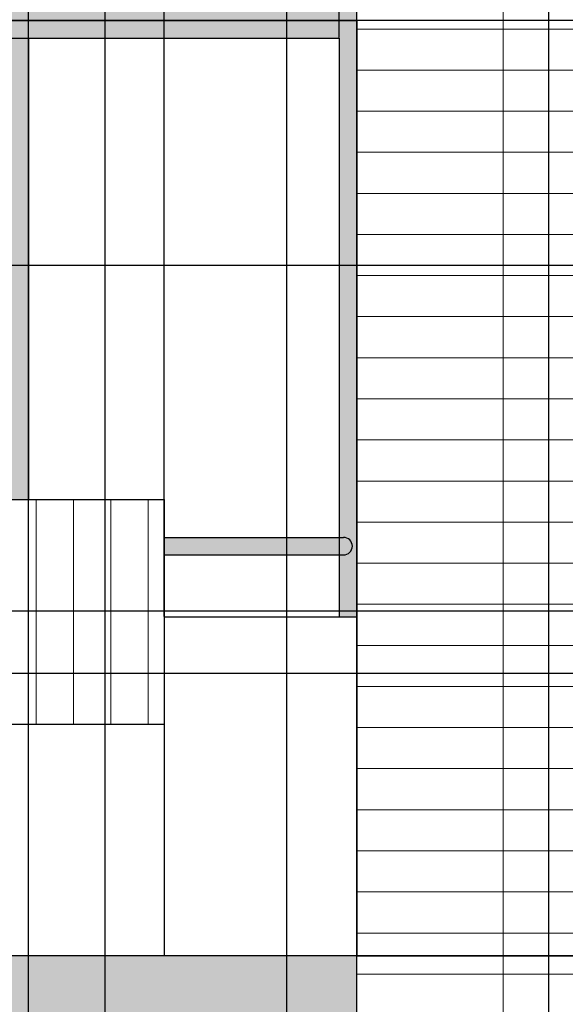
# Model space of a CAD drawing. Units: inches. Extents: x 241 to 943, y 109 to 1396.
# Tile 23 of 34: x 470 to 532, y 1065 to 1178. Entities that reach past the tile are written whole.
import ezdxf

# ---------------------------------------------------------------- set-up
doc = ezdxf.new("R2010")
doc.units = ezdxf.units.IN
doc.header["$MEASUREMENT"] = 0
for name, color, linetype, lineweight in [('A-ANNO-DIMS', 2, 'Continuous', 18), ('A-ELEV', 7, 'Continuous', 25), ('A-ELEV-SHAD', 9, 'Continuous', 13), ('A-GLAZ-PATT', 18, 'Continuous', 13), ('A-WALL-PATT', 8, 'Continuous', 13)]:
    doc.layers.add(name, color=color, linetype=linetype, lineweight=lineweight)
doc.styles.get("Standard").update_dxf_attribs({"font": 'arial.ttf'})
doc.dimstyles.get("Standard").update_dxf_attribs({"dimtxt": 1.4375, "dimasz": 0.18, "dimexe": 0.18, "dimexo": 0.0625, "dimgap": 0.09, "dimtad": 0, "dimtih": 1, "dimtoh": 1, "dimdec": 4, "dimzin": 0, "dimdsep": 46, "dimlunit": 4, "dimtxsty": 'Standard', "dimcen": 0.09, "dimadec": 0, "dimazin": 0, "dimtfac": 1, "dimtdec": 4, "dimtofl": 0, "dimtmove": 0, "dimatfit": 3, "dimfxl": 1, "dimtolj": 1, "dimtzin": 0, "dimarcsym": 0})

# ---------------------------------------------------------------- blocks, each defined once
blk = doc.blocks.new('BALCONY-RAIL')
for p, q in [((26.08, 26.37), (26.08, 52.06)), ((26.08, 52.06), (99.3, 52.06)), ((99.3, 52.06), (99.3, 26.37)), ((3.52, 47.73), (1, 47.73)), ((3.52, 47.73), (26.08, 47.73)), ((3.52, 45.73), (1, 45.73)), ((3.52, 45.73), (26.08, 45.73)), ((99.3, 26.37), (26.08, 26.37)), ((26.08, 26.37), (26.08, 0)), ((99.3, 26.37), (99.3, 0))]:
    blk.add_line(p, q)
blk.add_arc((1, 46.73), 1, 90, 270)
blk = doc.blocks.new('*D7')
at = {"layer": 'A-ANNO-DIMS', "color": 0, "lineweight": -2, "transparency": 16777216}
for p, q in [((508.24, 1336.12), (244.31, 1336.12)), ((244.49, 1335.94), (244.49, 753.25)), ((244.49, 168.92), (244.49, 751.6)), ((303.17, 168.74), (244.31, 168.74))]:
    blk.add_line(p, q, dxfattribs=at)
at = {"layer": 'A-ANNO-DIMS', "color": 0, "transparency": 16777216}
for points in [[(244.46, 1335.94), (244.52, 1335.94), (244.49, 1336.12)], [(244.46, 168.92), (244.52, 168.92), (244.49, 168.74)]]:
    blk.add_solid(points, dxfattribs=at)
at = {"layer": 'Defpoints', "color": 0, "transparency": 16777216}
for p in [(244.49, 1336.12), (508.31, 1336.12), (303.24, 168.74)]:
    blk.add_point(p, dxfattribs=at)
at = {"layer": 'A-ANNO-DIMS', "color": 0, "transparency": 16777216, "insert": (244.49, 752.43), "char_height": 1.438, "attachment_point": 5}
blk.add_mtext('\\A1;1167.4', dxfattribs=at)
blk = doc.blocks.new('*D10')
at = {"layer": 'A-ANNO-DIMS', "color": 0, "lineweight": -2, "transparency": 16777216}
for p, q in [((462.11, 384.24), (462.11, 1395.05)), ((462.29, 1394.87), (468.4, 1394.87)), ((479.42, 1394.87), (473.3, 1394.87)), ((479.6, 384.24), (479.6, 1395.05))]:
    blk.add_line(p, q, dxfattribs=at)
at = {"layer": 'A-ANNO-DIMS', "color": 0, "transparency": 16777216}
for points in [[(462.29, 1394.9), (462.29, 1394.84), (462.11, 1394.87)], [(479.42, 1394.9), (479.42, 1394.84), (479.6, 1394.87)]]:
    blk.add_solid(points, dxfattribs=at)
at = {"layer": 'Defpoints', "color": 0, "transparency": 16777216}
for p in [(479.6, 1394.87), (462.11, 384.18), (479.6, 384.18)]:
    blk.add_point(p, dxfattribs=at)
at = {"layer": 'A-ANNO-DIMS', "color": 0, "transparency": 16777216, "insert": (470.85, 1394.87), "char_height": 1.438, "attachment_point": 5}
blk.add_mtext('\\A1;17.49', dxfattribs=at)
blk = doc.blocks.new('*D11')
at = {"layer": 'A-ANNO-DIMS', "color": 0, "lineweight": -2, "transparency": 16777216}
for p, q in [((500.33, 384.24), (500.33, 1395.05)), ((500.51, 1394.87), (513.31, 1394.87)), ((530.05, 1394.87), (517.25, 1394.87)), ((530.23, 384.24), (530.23, 1395.05))]:
    blk.add_line(p, q, dxfattribs=at)
at = {"layer": 'A-ANNO-DIMS', "color": 0, "transparency": 16777216}
for points in [[(500.51, 1394.9), (500.51, 1394.84), (500.33, 1394.87)], [(530.05, 1394.9), (530.05, 1394.84), (530.23, 1394.87)]]:
    blk.add_solid(points, dxfattribs=at)
at = {"layer": 'Defpoints', "color": 0, "transparency": 16777216}
for p in [(530.23, 1394.87), (500.33, 384.18), (530.23, 384.18)]:
    blk.add_point(p, dxfattribs=at)
at = {"layer": 'A-ANNO-DIMS', "color": 0, "transparency": 16777216, "insert": (515.28, 1394.87), "char_height": 1.438, "attachment_point": 5}
blk.add_mtext('\\A1;29.9', dxfattribs=at)
blk = doc.blocks.new('*D12')
at = {"layer": 'A-ANNO-DIMS', "color": 0, "lineweight": -2, "transparency": 16777216}
for p, q in [((530.23, 384.24), (530.23, 1395.05)), ((530.41, 1394.87), (587.56, 1394.87)), ((650.73, 1394.87), (593.58, 1394.87)), ((650.91, 384.24), (650.91, 1395.05))]:
    blk.add_line(p, q, dxfattribs=at)
at = {"layer": 'A-ANNO-DIMS', "color": 0, "transparency": 16777216}
for points in [[(530.41, 1394.9), (530.41, 1394.84), (530.23, 1394.87)], [(650.73, 1394.9), (650.73, 1394.84), (650.91, 1394.87)]]:
    blk.add_solid(points, dxfattribs=at)
at = {"layer": 'Defpoints', "color": 0, "transparency": 16777216}
for p in [(650.91, 1394.87), (530.23, 384.18), (650.91, 384.18)]:
    blk.add_point(p, dxfattribs=at)
at = {"layer": 'A-ANNO-DIMS', "color": 0, "transparency": 16777216, "insert": (590.57, 1394.87), "char_height": 1.438, "attachment_point": 5}
blk.add_mtext('\\A1;120.68', dxfattribs=at)
blk = doc.blocks.new('*D49')
at = {"layer": 'A-ANNO-DIMS', "color": 0, "lineweight": -2, "transparency": 16777216}
for p, q in [((766.24, 1177.54), (244.31, 1177.54)), ((244.49, 1177.36), (244.49, 1141.12)), ((244.49, 1103.23), (244.49, 1139.47)), ((766.24, 1103.05), (244.31, 1103.05))]:
    blk.add_line(p, q, dxfattribs=at)
at = {"layer": 'A-ANNO-DIMS', "color": 0, "transparency": 16777216}
for points in [[(244.46, 1177.36), (244.52, 1177.36), (244.49, 1177.54)], [(244.46, 1103.23), (244.52, 1103.23), (244.49, 1103.05)]]:
    blk.add_solid(points, dxfattribs=at)
at = {"layer": 'Defpoints', "color": 0, "transparency": 16777216}
for p in [(244.49, 1177.54), (766.3, 1177.54), (766.3, 1103.05)]:
    blk.add_point(p, dxfattribs=at)
at = {"layer": 'A-ANNO-DIMS', "color": 0, "transparency": 16777216, "insert": (244.49, 1140.29), "char_height": 1.438, "attachment_point": 5}
blk.add_mtext('\\A1;74.49', dxfattribs=at)
blk = doc.blocks.new('*D57')
at = {"layer": 'A-ANNO-DIMS', "color": 0, "lineweight": -2, "transparency": 16777216}
for p, q in [((508.31, 1070.92), (508.31, 1395.05)), ((508.49, 1394.87), (518.04, 1394.87)), ((533.77, 1394.87), (524.21, 1394.87)), ((533.95, 1108.23), (533.95, 1395.05))]:
    blk.add_line(p, q, dxfattribs=at)
at = {"layer": 'A-ANNO-DIMS', "color": 0, "transparency": 16777216}
for points in [[(508.49, 1394.9), (508.49, 1394.84), (508.31, 1394.87)], [(533.77, 1394.9), (533.77, 1394.84), (533.95, 1394.87)]]:
    blk.add_solid(points, dxfattribs=at)
at = {"layer": 'Defpoints', "color": 0, "transparency": 16777216}
for p in [(533.95, 1394.87), (533.95, 1108.17), (508.31, 1070.85)]:
    blk.add_point(p, dxfattribs=at)
at = {"layer": 'A-ANNO-DIMS', "color": 0, "transparency": 16777216, "insert": (521.13, 1394.87), "char_height": 1.438, "attachment_point": 5}
blk.add_mtext('\\A1;25.646', dxfattribs=at)
blk = doc.blocks.new('*D59')
at = {"layer": 'A-ANNO-DIMS', "color": 0, "lineweight": -2, "transparency": 16777216}
for p, q in [((398.31, 1175.6), (398.31, 1395.05)), ((398.49, 1394.87), (450.7, 1394.87)), ((506.13, 1394.87), (453.92, 1394.87)), ((506.31, 1175.6), (506.31, 1395.05))]:
    blk.add_line(p, q, dxfattribs=at)
at = {"layer": 'A-ANNO-DIMS', "color": 0, "transparency": 16777216}
for points in [[(398.49, 1394.9), (398.49, 1394.84), (398.31, 1394.87)], [(506.13, 1394.9), (506.13, 1394.84), (506.31, 1394.87)]]:
    blk.add_solid(points, dxfattribs=at)
at = {"layer": 'Defpoints', "color": 0, "transparency": 16777216}
for p in [(506.31, 1394.87), (398.31, 1175.54), (506.31, 1175.54)]:
    blk.add_point(p, dxfattribs=at)
at = {"layer": 'A-ANNO-DIMS', "color": 0, "transparency": 16777216, "insert": (452.31, 1394.87), "char_height": 1.438, "attachment_point": 5}
blk.add_mtext('\\A1;108', dxfattribs=at)
blk = doc.blocks.new('*D62')
at = {"layer": 'A-ANNO-DIMS', "color": 0, "lineweight": -2, "transparency": 16777216}
for p, q in [((424.11, 568.89), (424.11, 1395.05)), ((424.29, 1394.87), (492.35, 1394.87)), ((565.02, 1394.87), (496.96, 1394.87)), ((565.2, 568.89), (565.2, 1395.05))]:
    blk.add_line(p, q, dxfattribs=at)
at = {"layer": 'A-ANNO-DIMS', "color": 0, "transparency": 16777216}
for points in [[(424.29, 1394.9), (424.29, 1394.84), (424.11, 1394.87)], [(565.02, 1394.9), (565.02, 1394.84), (565.2, 1394.87)]]:
    blk.add_solid(points, dxfattribs=at)
at = {"layer": 'Defpoints', "color": 0, "transparency": 16777216}
for p in [(565.2, 1394.87), (424.11, 568.83), (565.2, 568.83)]:
    blk.add_point(p, dxfattribs=at)
at = {"layer": 'A-ANNO-DIMS', "color": 0, "transparency": 16777216, "insert": (494.66, 1394.87), "char_height": 1.438, "attachment_point": 5}
blk.add_mtext('\\A1;141.1', dxfattribs=at)
blk = doc.blocks.new('*D65')
at = {"layer": 'A-ANNO-DIMS', "color": 0, "lineweight": -2, "transparency": 16777216}
for p, q in [((424.11, 700.85), (424.11, 1395.05)), ((424.29, 1394.87), (505.52, 1394.87)), ((592.77, 1394.87), (511.54, 1394.87)), ((592.95, 700.85), (592.95, 1395.05))]:
    blk.add_line(p, q, dxfattribs=at)
at = {"layer": 'A-ANNO-DIMS', "color": 0, "transparency": 16777216}
for points in [[(424.29, 1394.9), (424.29, 1394.84), (424.11, 1394.87)], [(592.77, 1394.9), (592.77, 1394.84), (592.95, 1394.87)]]:
    blk.add_solid(points, dxfattribs=at)
at = {"layer": 'Defpoints', "color": 0, "transparency": 16777216}
for p in [(592.95, 1394.87), (424.11, 700.79), (592.95, 700.79)]:
    blk.add_point(p, dxfattribs=at)
at = {"layer": 'A-ANNO-DIMS', "color": 0, "transparency": 16777216, "insert": (508.53, 1394.87), "char_height": 1.438, "attachment_point": 5}
blk.add_mtext('\\A1;168.85', dxfattribs=at)
blk = doc.blocks.new('*D67')
at = {"layer": 'A-ANNO-DIMS', "color": 0, "lineweight": -2, "transparency": 16777216}
for p, q in [((389.04, 773.55), (389.04, 1395.05)), ((389.22, 1394.87), (495.34, 1394.87)), ((607.64, 1394.87), (501.52, 1394.87)), ((607.82, 773.55), (607.82, 1395.05))]:
    blk.add_line(p, q, dxfattribs=at)
at = {"layer": 'A-ANNO-DIMS', "color": 0, "transparency": 16777216}
for points in [[(389.22, 1394.9), (389.22, 1394.84), (389.04, 1394.87)], [(607.64, 1394.9), (607.64, 1394.84), (607.82, 1394.87)]]:
    blk.add_solid(points, dxfattribs=at)
at = {"layer": 'Defpoints', "color": 0, "transparency": 16777216}
for p in [(607.82, 1394.87), (389.04, 773.49), (607.82, 773.49)]:
    blk.add_point(p, dxfattribs=at)
at = {"layer": 'A-ANNO-DIMS', "color": 0, "transparency": 16777216, "insert": (498.43, 1394.87), "char_height": 1.438, "attachment_point": 5}
blk.add_mtext('\\A1;218.77', dxfattribs=at)
blk = doc.blocks.new('*D69')
at = {"layer": 'A-ANNO-DIMS', "color": 0, "lineweight": -2, "transparency": 16777216}
for p, q in [((389.04, 941.55), (389.04, 1395.05)), ((389.22, 1394.87), (476.28, 1394.87)), ((567.95, 1394.87), (480.9, 1394.87)), ((568.13, 941.55), (568.13, 1395.05))]:
    blk.add_line(p, q, dxfattribs=at)
at = {"layer": 'A-ANNO-DIMS', "color": 0, "transparency": 16777216}
for points in [[(389.22, 1394.9), (389.22, 1394.84), (389.04, 1394.87)], [(567.95, 1394.9), (567.95, 1394.84), (568.13, 1394.87)]]:
    blk.add_solid(points, dxfattribs=at)
at = {"layer": 'Defpoints', "color": 0, "transparency": 16777216}
for p in [(568.13, 1394.87), (389.04, 941.49), (568.13, 941.49)]:
    blk.add_point(p, dxfattribs=at)
at = {"layer": 'A-ANNO-DIMS', "color": 0, "transparency": 16777216, "insert": (478.59, 1394.87), "char_height": 1.438, "attachment_point": 5}
blk.add_mtext('\\A1;179.1', dxfattribs=at)
blk = doc.blocks.new('*D72')
at = {"layer": 'A-ANNO-DIMS', "color": 0, "lineweight": -2, "transparency": 16777216}
for p, q in [((389.04, 1109.55), (389.04, 1395.05)), ((389.22, 1394.87), (435.74, 1394.87)), ((486.16, 1394.87), (439.65, 1394.87)), ((486.34, 1109.55), (486.34, 1395.05))]:
    blk.add_line(p, q, dxfattribs=at)
at = {"layer": 'A-ANNO-DIMS', "color": 0, "transparency": 16777216}
for points in [[(389.22, 1394.9), (389.22, 1394.84), (389.04, 1394.87)], [(486.16, 1394.9), (486.16, 1394.84), (486.34, 1394.87)]]:
    blk.add_solid(points, dxfattribs=at)
at = {"layer": 'Defpoints', "color": 0, "transparency": 16777216}
for p in [(486.34, 1394.87), (389.04, 1109.49), (486.34, 1109.49)]:
    blk.add_point(p, dxfattribs=at)
at = {"layer": 'A-ANNO-DIMS', "color": 0, "transparency": 16777216, "insert": (437.69, 1394.87), "char_height": 1.438, "attachment_point": 5}
blk.add_mtext('\\A1;97.3', dxfattribs=at)
blk = doc.blocks.new('*D79')
at = {"layer": 'A-ANNO-DIMS', "color": 0, "lineweight": -2, "transparency": 16777216}
for p, q in [((479.6, 384.24), (479.6, 1395.05)), ((479.78, 1394.87), (486.88, 1394.87)), ((500.15, 1394.87), (493.05, 1394.87)), ((500.33, 384.24), (500.33, 1395.05))]:
    blk.add_line(p, q, dxfattribs=at)
at = {"layer": 'A-ANNO-DIMS', "color": 0, "transparency": 16777216}
for points in [[(479.78, 1394.9), (479.78, 1394.84), (479.6, 1394.87)], [(500.15, 1394.9), (500.15, 1394.84), (500.33, 1394.87)]]:
    blk.add_solid(points, dxfattribs=at)
at = {"layer": 'Defpoints', "color": 0, "transparency": 16777216}
for p in [(500.33, 1394.87), (479.6, 384.18), (500.33, 384.18)]:
    blk.add_point(p, dxfattribs=at)
at = {"layer": 'A-ANNO-DIMS', "color": 0, "transparency": 16777216, "insert": (489.96, 1394.87), "char_height": 1.438, "attachment_point": 5}
blk.add_mtext('\\A1;20.736', dxfattribs=at)
blk = doc.blocks.new('*D89')
at = {"layer": 'A-ANNO-DIMS', "color": 0, "lineweight": -2, "transparency": 16777216}
for p, q in [((377.04, 841.6), (377.04, 1395.05)), ((377.22, 1394.87), (494.32, 1394.87)), ((617.58, 1394.87), (500.48, 1394.87)), ((617.76, 841.6), (617.76, 1395.05))]:
    blk.add_line(p, q, dxfattribs=at)
at = {"layer": 'A-ANNO-DIMS', "color": 0, "transparency": 16777216}
for points in [[(377.22, 1394.9), (377.22, 1394.84), (377.04, 1394.87)], [(617.58, 1394.9), (617.58, 1394.84), (617.76, 1394.87)]]:
    blk.add_solid(points, dxfattribs=at)
at = {"layer": 'Defpoints', "color": 0, "transparency": 16777216}
for p in [(617.76, 1394.87), (377.04, 841.54), (617.76, 841.54)]:
    blk.add_point(p, dxfattribs=at)
at = {"layer": 'A-ANNO-DIMS', "color": 0, "transparency": 16777216, "insert": (497.4, 1394.87), "char_height": 1.438, "attachment_point": 5}
blk.add_mtext('\\A1;240.72', dxfattribs=at)
blk = doc.blocks.new('*D92')
at = {"layer": 'A-ANNO-DIMS', "color": 0, "lineweight": -2, "transparency": 16777216}
for p, q in [((508.24, 1336.12), (244.31, 1336.12)), ((244.49, 1335.94), (244.49, 1204.31)), ((244.49, 1071.03), (244.49, 1202.66)), ((508.24, 1070.85), (244.31, 1070.85))]:
    blk.add_line(p, q, dxfattribs=at)
at = {"layer": 'A-ANNO-DIMS', "color": 0, "transparency": 16777216}
for points in [[(244.46, 1335.94), (244.52, 1335.94), (244.49, 1336.12)], [(244.46, 1071.03), (244.52, 1071.03), (244.49, 1070.85)]]:
    blk.add_solid(points, dxfattribs=at)
at = {"layer": 'Defpoints', "color": 0, "transparency": 16777216}
for p in [(244.49, 1336.12), (508.31, 1336.12), (508.31, 1070.85)]:
    blk.add_point(p, dxfattribs=at)
at = {"layer": 'A-ANNO-DIMS', "color": 0, "transparency": 16777216, "insert": (244.49, 1203.48), "char_height": 1.438, "attachment_point": 5}
blk.add_mtext('\\A1;265.26', dxfattribs=at)
blk = doc.blocks.new('*D95')
at = {"layer": 'A-ANNO-DIMS', "color": 0, "lineweight": -2, "transparency": 16777216}
for p, q in [((724.88, 1108.17), (940.6, 1108.17)), ((940.42, 1107.99), (940.42, 1090.34)), ((940.42, 1071.03), (940.42, 1088.69)), ((508.37, 1070.85), (940.6, 1070.85))]:
    blk.add_line(p, q, dxfattribs=at)
at = {"layer": 'A-ANNO-DIMS', "color": 0, "transparency": 16777216}
for points in [[(940.39, 1107.99), (940.45, 1107.99), (940.42, 1108.17)], [(940.39, 1071.03), (940.45, 1071.03), (940.42, 1070.85)]]:
    blk.add_solid(points, dxfattribs=at)
at = {"layer": 'Defpoints', "color": 0, "transparency": 16777216}
for p in [(724.82, 1108.17), (940.42, 1108.17), (508.31, 1070.85)]:
    blk.add_point(p, dxfattribs=at)
at = {"layer": 'A-ANNO-DIMS', "color": 0, "transparency": 16777216, "insert": (940.42, 1089.51), "char_height": 1.438, "attachment_point": 5}
blk.add_mtext('\\A1;37.315', dxfattribs=at)
blk = doc.blocks.new('*D99')
at = {"layer": 'A-ANNO-DIMS', "color": 0, "lineweight": -2, "transparency": 16777216}
for p, q in [((417.09, 181.71), (417.09, 1395.05)), ((417.27, 1394.87), (539.16, 1394.87)), ((667.21, 1394.87), (545.33, 1394.87)), ((667.39, 214.58), (667.39, 1395.05))]:
    blk.add_line(p, q, dxfattribs=at)
at = {"layer": 'A-ANNO-DIMS', "color": 0, "transparency": 16777216}
for points in [[(417.27, 1394.9), (417.27, 1394.84), (417.09, 1394.87)], [(667.21, 1394.9), (667.21, 1394.84), (667.39, 1394.87)]]:
    blk.add_solid(points, dxfattribs=at)
at = {"layer": 'Defpoints', "color": 0, "transparency": 16777216}
for p in [(667.39, 1394.87), (667.39, 214.52), (417.09, 181.65)]:
    blk.add_point(p, dxfattribs=at)
at = {"layer": 'A-ANNO-DIMS', "color": 0, "transparency": 16777216, "insert": (542.24, 1394.87), "char_height": 1.438, "attachment_point": 5}
blk.add_mtext('\\A1;250.30', dxfattribs=at)
blk = doc.blocks.new('*D103')
at = {"layer": 'A-ANNO-DIMS', "color": 0, "lineweight": -2, "transparency": 16777216}
for p, q in [((470.87, 1007.6), (470.87, 1395.05)), ((471.05, 1394.87), (487.08, 1394.87)), ((508.13, 1394.87), (492.1, 1394.87)), ((508.31, 1009.6), (508.31, 1395.05))]:
    blk.add_line(p, q, dxfattribs=at)
at = {"layer": 'A-ANNO-DIMS', "color": 0, "transparency": 16777216}
for points in [[(471.05, 1394.9), (471.05, 1394.84), (470.87, 1394.87)], [(508.13, 1394.9), (508.13, 1394.84), (508.31, 1394.87)]]:
    blk.add_solid(points, dxfattribs=at)
at = {"layer": 'Defpoints', "color": 0, "transparency": 16777216}
for p in [(508.31, 1394.87), (508.31, 1009.54), (470.87, 1007.54)]:
    blk.add_point(p, dxfattribs=at)
at = {"layer": 'A-ANNO-DIMS', "color": 0, "transparency": 16777216, "insert": (489.59, 1394.87), "char_height": 1.438, "attachment_point": 5}
blk.add_mtext('\\A1;37.44', dxfattribs=at)
blk = doc.blocks.new('*D110')
at = {"layer": 'A-ANNO-DIMS', "color": 0, "lineweight": -2, "transparency": 16777216}
for p, q in [((535.89, 1149.58), (244.31, 1149.58)), ((244.49, 1149.4), (244.49, 1130.7)), ((244.49, 1110.35), (244.49, 1129.05)), ((535.89, 1110.17), (244.31, 1110.17))]:
    blk.add_line(p, q, dxfattribs=at)
at = {"layer": 'A-ANNO-DIMS', "color": 0, "transparency": 16777216}
for points in [[(244.46, 1149.4), (244.52, 1149.4), (244.49, 1149.58)], [(244.46, 1110.35), (244.52, 1110.35), (244.49, 1110.17)]]:
    blk.add_solid(points, dxfattribs=at)
at = {"layer": 'Defpoints', "color": 0, "transparency": 16777216}
for p in [(244.49, 1149.58), (535.95, 1149.58), (535.95, 1110.17)]:
    blk.add_point(p, dxfattribs=at)
at = {"layer": 'A-ANNO-DIMS', "color": 0, "transparency": 16777216, "insert": (244.49, 1129.87), "char_height": 1.438, "attachment_point": 5}
blk.add_mtext('\\A1;39.41', dxfattribs=at)

msp = doc.modelspace()

# ---------------------------------------------------------------- hatches: boundary and pattern name
at = {"layer": 'A-ELEV-SHAD'}
h = msp.add_hatch(color=256, dxfattribs=at)
h.dxf.hatch_style = 1
h.paths.add_polyline_path([(508.3064, 1070.8538), (377.0391, 1070.8538), (377.0391, 1009.5382), (508.3064, 1009.5382)])
h.paths.add_polyline_path([(508.3064, 1238.8538), (377.0391, 1238.8538), (377.0391, 1177.5382), (508.3064, 1177.5382)])
h.paths.add_polyline_path([(581.3632, 902.8538), (568.1348, 902.8538), (553.5166, 902.8538), (377.0391, 902.8538), (377.0391, 841.5382), (553.5166, 841.5382), (564.8076, 841.5382), (581.3632, 841.5382)])
h.paths.add_polyline_path([(820.8374, 1275.9142), (747.7579, 1275.9142), (747.7579, 1238.8538), (820.8374, 1238.8538)])
h.paths.add_polyline_path([(820.8374, 1238.8538), (747.7579, 1238.8538), (747.9341, 1223.0633), (820.8374, 1223.0633)])
h.paths.add_polyline_path([(396.3125, 841.5382), (377.0391, 841.5382), (377.0391, 734.8538), (389.0429, 734.8538), (389.0429, 735.188), (389.0429, 773.4916), (396.3125, 773.4916), (396.3125, 780.5808), (390.5597, 780.5808), (388.0428, 780.5808, -1), (388.0428, 782.5808), (390.5597, 782.5808), (396.3125, 782.5808)])
h = msp.add_hatch(color=256, dxfattribs=at)
h.dxf.hatch_style = 1
h.paths.add_polyline_path([(537.4269, 698.7912), (534.1778, 698.7912), (534.1778, 659.3434), (537.4269, 659.3434)])
h.paths.add_polyline_path([(508.0803, 698.7912), (450.9259, 698.7912), (450.9259, 659.3434), (452.9259, 659.3434), (452.9259, 696.7912), (506.0803, 696.7912), (506.0803, 659.3434), (508.0803, 659.3434)])
h.paths.add_polyline_path([(481.5031, 696.7912), (479.5031, 696.7912), (479.5031, 659.3434), (481.5031, 659.3434)], flags=17)
h.paths.add_polyline_path([(481.5031, 657.3434), (479.5031, 657.3434), (479.5031, 653.3371), (481.5031, 653.3371)], flags=17)
h.paths.add_polyline_path([(508.0803, 657.3434), (506.0803, 657.3434), (506.0803, 653.3371), (452.9259, 653.3371), (452.9259, 657.3434), (450.9259, 657.3434), (450.9259, 651.3371), (508.0803, 651.3371)])
h.paths.add_polyline_path([(428.1173, 839.5382), (426.1173, 839.5382), (426.1173, 786.9154), (428.1173, 786.9154)], flags=17)
h.paths.add_polyline_path([(470.8692, 839.5382), (468.8692, 839.5382), (468.8692, 786.9154), (470.8692, 786.9154)], flags=17)
h.paths.add_polyline_path([(508.3064, 841.5382), (396.3125, 841.5382), (396.3125, 782.5808), (398.3125, 782.5808), (398.3125, 839.5382), (506.3064, 839.5382), (506.3064, 782.5808), (508.3064, 782.5808)])
h.paths.add_polyline_path([(398.3125, 780.5808), (396.3125, 780.5808), (396.3125, 773.4916), (398.3125, 773.4916)])
h.paths.add_polyline_path([(508.3064, 780.5808), (506.3064, 780.5808), (506.3064, 773.4916), (508.3064, 773.4916)])
h.paths.add_polyline_path([(715.6236, 841.5382), (678.2674, 841.5382), (678.2674, 734.8538), (715.6236, 734.8538)])
h.paths.add_polyline_path([(680.2674, 839.5382), (682.4526, 839.5382), (713.6236, 839.5382), (713.6236, 736.9235), (690.2047, 736.9235), (680.2674, 736.9235)], flags=16)
h.paths.add_polyline_path([(792.691, 841.5382), (747.7579, 841.5382), (747.7579, 734.8538), (754.5373, 734.8538), (754.5373, 736.9235), (754.5373, 839.5382), (756.7224, 839.5382), (787.8934, 839.5382), (787.8934, 765.9585), (792.691, 765.9585)])
h.paths.add_polyline_path([(659.2925, 1009.5382), (657.2925, 1009.5382), (657.2925, 902.8538), (659.2925, 902.8538)])
h.paths.add_polyline_path([(751.5078, 976.6275), (712.5839, 976.6275), (712.5839, 974.6275), (751.5078, 974.6275)])
h.paths.add_polyline_path([(470.8692, 1007.5382), (468.8692, 1007.5382), (468.8692, 954.9154), (470.8692, 954.9154)], flags=17)
h.paths.add_polyline_path([(508.3064, 1009.5382), (396.3125, 1009.5382), (396.3125, 950.5808), (398.3125, 950.5808), (398.3125, 1007.5382), (506.3064, 1007.5382), (506.3064, 950.5808), (508.3064, 950.5808)])
h.paths.add_polyline_path([(428.1173, 1007.5382), (426.1173, 1007.5382), (426.1173, 954.9154), (428.1173, 954.9154)], flags=17)
h.paths.add_polyline_path([(398.3125, 948.5808), (396.3125, 948.5808), (396.3125, 941.4916), (398.3125, 941.4916)])
h.paths.add_polyline_path([(508.3064, 948.5808), (506.3064, 948.5808), (506.3064, 941.4916), (508.3064, 941.4916)])
h.paths.add_polyline_path([(428.1173, 1175.5382), (426.1173, 1175.5382), (426.1173, 1122.9154), (428.1173, 1122.9154)], flags=17)
h.paths.add_polyline_path([(508.3064, 1177.5382), (396.3125, 1177.5382), (396.3125, 1118.5808), (398.3125, 1118.5808), (398.3125, 1175.5382), (506.3064, 1175.5382), (506.3064, 1118.5808), (506.8039, 1118.5808, -1), (506.8039, 1116.5808), (506.3064, 1116.5808), (506.3064, 1109.4916), (508.3064, 1109.4916)])
h.paths.add_polyline_path([(470.8692, 1175.5382), (468.8692, 1175.5382), (468.8692, 1122.9154), (470.8692, 1122.9154)], flags=17)
h.paths.add_polyline_path([(398.3125, 1116.5808), (396.3125, 1116.5808), (396.3125, 1109.4916), (398.3125, 1109.4916)], flags=17)
h.paths.add_polyline_path([(724.819, 1177.7336), (533.952, 1177.7336), (533.952, 1108.1686), (724.819, 1108.1686)])
h.paths.add_polyline_path([(535.952, 1175.7336), (722.819, 1175.7336), (722.819, 1110.1686), (535.952, 1110.1686)], flags=0)
h.paths.add_polyline_path([(622.521, 1136.0739), (643.4534, 1136.0739), (643.4534, 1134.0739), (622.521, 1134.0739)], flags=0)
h.paths.add_polyline_path([(722.819, 1175.7336), (535.952, 1175.7336), (535.952, 1110.1686), (722.819, 1110.1686)], flags=16)
h.paths.add_polyline_path([(565.947, 1151.5772), (535.952, 1151.5772), (535.952, 1149.5772), (565.947, 1149.5772)], flags=0)
at = {"layer": 'A-GLAZ-PATT'}
h = msp.add_hatch(dxfattribs=at)
h.set_pattern_fill('ANSI31', color=256, scale=34, angle=45)
h.paths.add_polyline_path([(486.3418, 786.9154), (413.1187, 786.9154), (413.1187, 761.2284), (486.3418, 761.2284)])
h.paths.add_polyline_path([(486.3418, 954.9154), (413.1187, 954.9154), (413.1187, 929.2284), (486.3418, 929.2284)])
h.paths.add_polyline_path([(462.1074, 289.6933), (390.895, 289.6933), (390.895, 277.4626), (390.895, 274.3507), (462.1074, 274.3507), (462.1074, 277.4626)])
h.paths.add_polyline_path([(500.3323, 289.6933), (479.596, 289.6933), (479.596, 274.3507), (500.3323, 274.3507)])
h.paths.add_polyline_path([(450.9259, 566.8295), (426.1086, 566.8295), (426.1086, 498.4395), (446.4348, 498.4395), (446.4348, 519.3754), (450.9259, 519.3754), (450.9259, 525.3816), (445.5808, 525.3816, -1), (445.5808, 527.3816), (450.9259, 527.3816)])
h.paths.add_polyline_path([(563.2023, 508.9074), (534.1778, 508.9074), (508.1906, 508.9074), (508.1906, 498.4395), (563.2023, 498.4395)])
h.paths.add_polyline_path([(747.6328, 700.7912), (712.0171, 700.7912), (712.0171, 628.4013), (747.6328, 628.4013)])
h.paths.add_polyline_path([(446.4348, 643.7483), (426.1086, 643.7483), (426.1086, 630.4013), (446.4348, 630.4013)])
h.paths.add_polyline_path([(564.8076, 841.5382), (553.5166, 841.5382), (508.3064, 841.5382), (508.3064, 782.5808), (564.8076, 782.5808)])
h.paths.add_polyline_path([(564.8076, 780.5808), (508.3064, 780.5808), (508.3064, 773.4916), (564.8076, 773.4916)])
h.paths.add_polyline_path([(792.691, 762.5799), (759.6248, 762.5799), (759.6248, 736.9235), (759.6248, 734.8538), (792.691, 734.8538)])
h.paths.add_polyline_path([(564.8076, 1009.5382), (553.5166, 1009.5382), (508.3064, 1009.5382), (508.3064, 950.5808), (562.3033, 950.5808, -1), (562.3033, 948.5808), (508.3064, 948.5808), (508.3064, 941.4916), (564.8076, 941.4916)])
h.paths.add_polyline_path([(486.3418, 1122.9154), (413.1187, 1122.9154), (413.1187, 1097.2284), (486.3418, 1097.2284)])
h = msp.add_hatch(color=256, dxfattribs=at)
h.dxf.hatch_style = 1
h.paths.add_polyline_path([(396.3125, 1118.5808), (390.5597, 1118.5808), (388.0428, 1118.5808, 1), (388.0428, 1116.5808), (390.5597, 1116.5808), (396.3125, 1116.5808)])
h.paths.add_polyline_path([(398.3125, 1118.5808), (396.3125, 1118.5808), (396.3125, 1116.5808), (398.3125, 1116.5808)])
h.paths.add_polyline_path([(413.1187, 1118.5808), (398.3125, 1118.5808), (398.3125, 1116.5808), (413.1187, 1116.5808)])
h.paths.add_polyline_path([(506.3064, 1118.5808), (486.3418, 1118.5808), (486.3418, 1116.5808), (506.3064, 1116.5808)])
h.paths.add_polyline_path([(506.8039, 1118.5808), (506.3064, 1118.5808), (506.3064, 1116.5808), (506.8039, 1116.5808, 1)])
h.paths.add_polyline_path([(396.3125, 950.5808), (390.5597, 950.5808), (388.0428, 950.5808, 1), (388.0428, 948.5808), (390.5597, 948.5808), (396.3125, 948.5808)])
h.paths.add_polyline_path([(398.3125, 950.5808), (396.3125, 950.5808), (396.3125, 948.5808), (398.3125, 948.5808)])
h.paths.add_polyline_path([(413.1187, 950.5808), (398.3125, 950.5808), (398.3125, 948.5808), (413.1187, 948.5808)])
h.paths.add_polyline_path([(506.3064, 950.5808), (486.3418, 950.5808), (486.3418, 948.5808), (506.3064, 948.5808)])
h.paths.add_polyline_path([(508.3064, 950.5808), (506.3064, 950.5808), (506.3064, 948.5808), (508.3064, 948.5808)])
h.paths.add_polyline_path([(562.3033, 950.5808), (508.3064, 950.5808), (508.3064, 948.5808), (562.3033, 948.5808, 1)])
h.paths.add_polyline_path([(396.3125, 782.5808), (390.5597, 782.5808), (388.0428, 782.5808, 1), (388.0428, 780.5808), (390.5597, 780.5808), (396.3125, 780.5808)])
h.paths.add_polyline_path([(398.3125, 782.5808), (396.3125, 782.5808), (396.3125, 780.5808), (398.3125, 780.5808)])
h.paths.add_polyline_path([(413.1187, 782.5808), (398.3125, 782.5808), (398.3125, 780.5808), (413.1187, 780.5808)])
h.paths.add_polyline_path([(506.3064, 782.5808), (486.3418, 782.5808), (486.3418, 780.5808), (506.3064, 780.5808)])
h.paths.add_polyline_path([(508.3064, 782.5808), (506.3064, 782.5808), (506.3064, 780.5808), (508.3064, 780.5808)])
h.paths.add_polyline_path([(564.8076, 782.5808), (508.3064, 782.5808), (508.3064, 780.5808), (564.8076, 780.5808)])
h.paths.add_polyline_path([(605.9087, 782.5808), (564.8076, 782.5808), (564.8076, 780.5808), (605.9087, 780.5808, 1)])
h.paths.add_polyline_path([(450.9259, 659.3434), (445.5808, 659.3434, 1), (445.5808, 657.3434), (450.9259, 657.3434)])
h.paths.add_polyline_path([(452.9259, 659.3434), (450.9259, 659.3434), (450.9259, 657.3434), (452.9259, 657.3434)])
h.paths.add_polyline_path([(506.0803, 659.3434), (452.9259, 659.3434), (452.9259, 657.3434), (506.0803, 657.3434)])
h.paths.add_polyline_path([(508.0803, 659.3434), (506.0803, 659.3434), (506.0803, 657.3434), (508.0803, 657.3434)])
h.paths.add_polyline_path([(563.2023, 659.3434), (537.4269, 659.3434), (537.4269, 657.3434), (563.2023, 657.3434)])
h.paths.add_polyline_path([(590.8792, 659.3434), (563.9297, 659.3434), (563.9297, 657.3434), (590.8792, 657.3434)])
h.paths.add_polyline_path([(563.9297, 659.3434), (563.2023, 659.3434), (563.2023, 657.3434), (563.9297, 657.3434)])
h.paths.add_polyline_path([(537.4269, 659.3434), (534.1778, 659.3434), (534.1778, 657.3434), (537.4269, 657.3434)])
h.paths.add_polyline_path([(534.1778, 659.3434), (508.0803, 659.3434), (508.0803, 657.3434), (534.1778, 657.3434)])
h.paths.add_polyline_path([(450.9259, 527.3816), (445.5808, 527.3816, 1), (445.5808, 525.3816), (450.9259, 525.3816)])
h.paths.add_polyline_path([(452.9259, 527.3816), (450.9259, 527.3816), (450.9259, 525.3816), (452.9259, 525.3816)])
h.paths.add_polyline_path([(479.5031, 527.3816), (452.9259, 527.3816), (452.9259, 525.3816), (479.5031, 525.3816)])
h.paths.add_polyline_path([(481.5031, 527.3816), (479.5031, 527.3816), (479.5031, 525.3816), (481.5031, 525.3816)])
h.paths.add_polyline_path([(506.0803, 527.3816), (481.5031, 527.3816), (481.5031, 525.3816), (506.0803, 525.3816)])
h.paths.add_polyline_path([(508.0803, 527.3816), (506.0803, 527.3816), (506.0803, 525.3816), (508.0803, 525.3816)])
h.paths.add_polyline_path([(563.2023, 527.3816), (508.0803, 527.3816), (508.0803, 525.3816), (563.2023, 525.3816)])
at = {"layer": 'A-WALL-PATT'}
h = msp.add_hatch(dxfattribs=at)
h.set_pattern_fill('GRATE', color=256, scale=150)
h.paths.add_polyline_path([(747.7579, 1238.8538), (747.7579, 1275.9142), (747.7579, 1336.1154), (508.3064, 1336.1154), (508.3064, 1275.9142), (508.3064, 1238.8538), (508.3064, 1177.5382), (508.3064, 1109.4916), (508.3064, 1070.8538), (553.5166, 1070.8538), (749.6328, 1070.8538)])
h.paths.add_polyline_path([(533.952, 1108.1686), (533.952, 1177.7336), (533.952, 1303.0286), (724.819, 1303.0286), (724.819, 1108.1686)], flags=16)
h.paths.add_polyline_path([(535.952, 1110.1686), (535.952, 1175.7336), (722.819, 1175.7336), (722.819, 1110.1686)], flags=0)
h.paths.add_polyline_path([(643.4534, 1134.0739), (622.521, 1134.0739), (622.521, 1136.0739), (643.4534, 1136.0739)], flags=0)
h.paths.add_polyline_path([(617.7594, 568.8295), (617.7594, 734.8538), (377.0391, 734.8538), (377.0391, 566.8538), (377.0391, 400.8295), (417.0913, 400.8295), (618.9643, 400.8295)])
h.paths.add_polyline_path([(424.1086, 496.4395), (424.1086, 568.8295), (565.2023, 568.8295), (565.2023, 496.4395)], flags=16)
h.paths.add_polyline_path([(426.1086, 498.4395), (426.1086, 566.8295), (563.2023, 566.8295), (563.2023, 508.9074), (563.2023, 498.4395)], flags=0)
h.paths.add_polyline_path([(508.0803, 508.9074), (508.0803, 519.3754), (450.9259, 519.3754), (450.9259, 525.3816), (445.5808, 525.3816, -1), (445.5808, 527.3816), (450.9259, 527.3816), (450.9259, 566.8295), (508.0803, 566.8295), (537.4269, 566.8295), (537.4269, 508.9074)], flags=0)
h.paths.add_polyline_path([(506.0803, 521.3754), (452.9259, 521.3754), (452.9259, 564.8295), (506.0803, 564.8295)], flags=0)
h.paths.add_polyline_path([(424.1086, 628.4013), (424.1086, 700.7912), (592.9542, 700.7912), (592.9542, 628.4013)], flags=16)
h.paths.add_polyline_path([(426.1086, 630.4013), (426.1086, 698.7912), (590.8792, 698.7912), (590.8792, 630.4013)], flags=0)
h.paths.add_polyline_path([(508.1906, 651.3371), (508.0803, 651.3371), (450.9259, 651.3371), (428.0291, 651.3371), (428.0291, 698.7912), (451.9767, 698.7912), (508.0803, 698.7912), (537.4269, 698.7912), (563.2023, 698.7912), (563.2023, 659.3434), (563.9297, 659.3434), (563.9297, 651.3371)], flags=0)
h.paths.add_polyline_path([(506.0803, 653.3371), (452.9259, 653.3371), (452.9259, 657.3434), (445.5808, 657.3434, -1), (445.5808, 659.3434), (452.9259, 659.3434), (452.9259, 696.7912), (506.0803, 696.7912)], flags=0)
h = msp.add_hatch(dxfattribs=at)
h.set_pattern_fill('GRATE', color=256, scale=150)
h.paths.add_polyline_path([(820.8374, 1070.8538), (749.6328, 1070.8538), (553.5166, 1070.8538), (508.3064, 1070.8538), (508.3064, 1009.5382), (553.5166, 1009.5382), (564.8076, 1009.5382), (603.8694, 1009.5382), (751.5078, 1009.5382), (751.5078, 902.8538), (603.8694, 902.8538), (603.8694, 1009.5382), (564.8076, 1009.5382), (564.8076, 941.4916), (568.1348, 941.4916), (568.1348, 902.8538), (581.3632, 902.8538), (581.3632, 841.5382), (564.8076, 841.5382), (564.8076, 782.5808), (605.9087, 782.5808, -1), (605.9087, 780.5808), (564.8076, 780.5808), (564.8076, 773.4916), (597.514, 773.4916), (607.8162, 773.4916), (607.8162, 734.8538), (617.7594, 734.8538), (617.7594, 841.5382), (792.691, 841.5382), (792.691, 734.8538), (617.7594, 734.8538), (617.7594, 702.7912), (749.6328, 702.7912), (749.6328, 626.4013), (617.7594, 626.4013), (617.7594, 568.8295), (820.8374, 568.8295), (820.8374, 736.8295), (820.8374, 902.8538)])

# ---------------------------------------------------------------- linework, layer by layer
at = {"layer": 'A-ELEV'}
for p, q in [((508.3064, 1177.5382), (508.3064, 1238.8538)), ((377.0391, 1177.5382), (508.3064, 1177.5382)), ((508.3064, 1177.5382), (508.3064, 1109.4916)), ((398.3125, 1175.5382), (506.3064, 1175.5382)), ((470.8692, 1175.5382), (470.8692, 1122.9154)), ((506.3064, 1175.5382), (506.3064, 1109.4916)), ((486.3418, 1118.5808), (506.8039, 1118.5808)), ((486.3418, 1116.5808), (506.8039, 1116.5808)), ((508.3064, 1109.4916), (486.3418, 1109.4916)), ((508.3064, 1109.4916), (508.3064, 1070.8538)), ((553.5166, 1070.8538), (377.0391, 1070.8538)), ((508.3064, 1009.5382), (508.3064, 1070.8538))]:
    msp.add_line(p, q, dxfattribs=at)
msp.add_arc((506.8039, 1117.5808), 1, 270, 90, dxfattribs=at)

# ---------------------------------------------------------------- block references
msp.add_blockref('BALCONY-RAIL', (387.043, 1070.854), dxfattribs=at)

# ---------------------------------------------------------------- dimensions: what is measured, and where the dimension line sits
at = {"layer": 'A-ANNO-DIMS'}
for base, p1, p2, override, picture, middle in [((617.7594, 1394.8654), (377.0391, 841.5382), (617.7594, 841.5382), {"dimdec": 2, "dimlfac": 1, "dimrnd": 0, "dimzin": 0, "dimdsep": 46, "dimlunit": 2}, '*D89', (497.3993, 1394.8654)), ((607.8162, 1394.8654), (389.0429, 773.4916), (607.8162, 773.4916), {"dimdec": 2, "dimlfac": 1, "dimrnd": 0, "dimzin": 0, "dimdsep": 46, "dimlunit": 2}, '*D67', (498.4295, 1394.8654)), ((568.1348, 1394.8654), (389.0429, 941.4916), (568.1348, 941.4916), {"dimdec": 1, "dimlfac": 1, "dimrnd": 0, "dimzin": 0, "dimdsep": 46, "dimlunit": 2}, '*D69', (478.5888, 1394.8654)), ((486.3418, 1394.8654), (389.0429, 1109.4916), (486.3418, 1109.4916), {"dimdec": 1, "dimlfac": 1, "dimrnd": 0, "dimzin": 0, "dimdsep": 46, "dimlunit": 2}, '*D72', (437.6924, 1394.8654)), ((506.3064, 1394.8654), (398.3125, 1175.5382), (506.3064, 1175.5382), {"dimdec": 0, "dimlfac": 1, "dimrnd": 0, "dimzin": 0, "dimdsep": 46, "dimlunit": 2}, '*D59', (452.3095, 1394.8654)), ((667.3935, 1394.8654), (417.0913, 181.649), (667.3935, 214.5189), {"dimdec": 2, "dimlfac": 1, "dimrnd": 0, "dimzin": 0, "dimdsep": 46, "dimlunit": 2}, '*D99', (542.2424, 1394.8654)), ((565.2023, 1394.8654), (424.1086, 568.8295), (565.2023, 568.8295), {"dimdec": 1, "dimlfac": 1, "dimrnd": 0, "dimzin": 0, "dimdsep": 46, "dimlunit": 2}, '*D62', (494.6554, 1394.8654)), ((592.9542, 1394.8654), (424.1086, 700.7912), (592.9542, 700.7912), {"dimdec": 2, "dimlfac": 1, "dimrnd": 0, "dimzin": 0, "dimdsep": 46, "dimlunit": 2}, '*D65', (508.5314, 1394.8654)), ((479.596, 1394.8654), (462.1074, 384.1784), (479.596, 384.1784), {"dimdec": 2, "dimlfac": 1, "dimrnd": 0, "dimzin": 0, "dimdsep": 46, "dimlunit": 2}, '*D10', (470.8517, 1394.8654)), ((508.3064, 1394.8654), (470.8692, 1007.5382), (508.3064, 1009.5382), {"dimdec": 2, "dimlfac": 1, "dimrnd": 0, "dimzin": 0, "dimdsep": 46, "dimlunit": 2}, '*D103', (489.5878, 1394.8654)), ((500.3323, 1394.8654), (479.596, 384.1784), (500.3323, 384.1784), {"dimdec": 3, "dimlfac": 1, "dimrnd": 0, "dimzin": 0, "dimdsep": 46, "dimlunit": 2}, '*D79', (489.9641, 1394.8654)), ((530.2303, 1394.8654), (500.3323, 384.1784), (530.2303, 384.1784), {"dimdec": 1, "dimlfac": 1, "dimrnd": 0, "dimzin": 0, "dimdsep": 46, "dimlunit": 2}, '*D11', (515.2813, 1394.8654)), ((533.952, 1394.8654), (508.3064, 1070.8538), (533.952, 1108.1686), {"dimdec": 3, "dimlfac": 1, "dimrnd": 0, "dimzin": 0, "dimdsep": 46, "dimlunit": 2}, '*D57', (521.1292, 1394.8654)), ((650.907, 1394.8654), (530.2303, 384.1784), (650.907, 384.1784), {"dimdec": 2, "dimlfac": 1, "dimrnd": 0, "dimzin": 0, "dimdsep": 46, "dimlunit": 2}, '*D12', (590.5686, 1394.8654))]:
    dim = msp.add_linear_dim(base=base, p1=p1, p2=p2, dimstyle='Standard', override=override, dxfattribs=at)
    dim.commit()
    dim.dimension.update_dxf_attribs({"geometry": picture, "text_midpoint": middle})
for base, p1, p2, override, picture, middle in [((244.4858, 1336.1154), (303.2358, 168.7407), (508.3064, 1336.1154), {"dimdec": 1, "dimlfac": 1, "dimrnd": 0, "dimzin": 0, "dimdsep": 46, "dimlunit": 2}, '*D7', (244.4858, 752.4281)), ((244.4858, 1336.1154), (508.3064, 1070.8538), (508.3064, 1336.1154), {"dimdec": 2, "dimlfac": 1, "dimrnd": 0, "dimzin": 0, "dimdsep": 46, "dimlunit": 2}, '*D92', (244.4858, 1203.4846)), ((244.4858, 1177.5382), (766.3038, 1103.0477), (766.3038, 1177.5382), {"dimdec": 2, "dimlfac": 1, "dimrnd": 0, "dimzin": 0, "dimdsep": 46, "dimlunit": 2}, '*D49', (244.4858, 1140.2929)), ((244.4858, 1149.5772), (535.952, 1110.1686), (535.952, 1149.5772), {"dimdec": 2, "dimlfac": 1, "dimrnd": 0, "dimzin": 0, "dimdsep": 46, "dimlunit": 2}, '*D110', (244.4858, 1129.8729)), ((940.417, 1108.1686), (508.3064, 1070.8538), (724.819, 1108.1686), {"dimdec": 3, "dimlfac": 1, "dimrnd": 0, "dimzin": 0, "dimdsep": 46, "dimlunit": 2}, '*D95', (940.417, 1089.5112))]:
    dim = msp.add_linear_dim(base=base, p1=p1, p2=p2, angle=90, dimstyle='Standard', override=override, dxfattribs=at)
    dim.commit()
    dim.dimension.update_dxf_attribs({"geometry": picture, "text_midpoint": middle})

doc.saveas('drawing.dxf')
